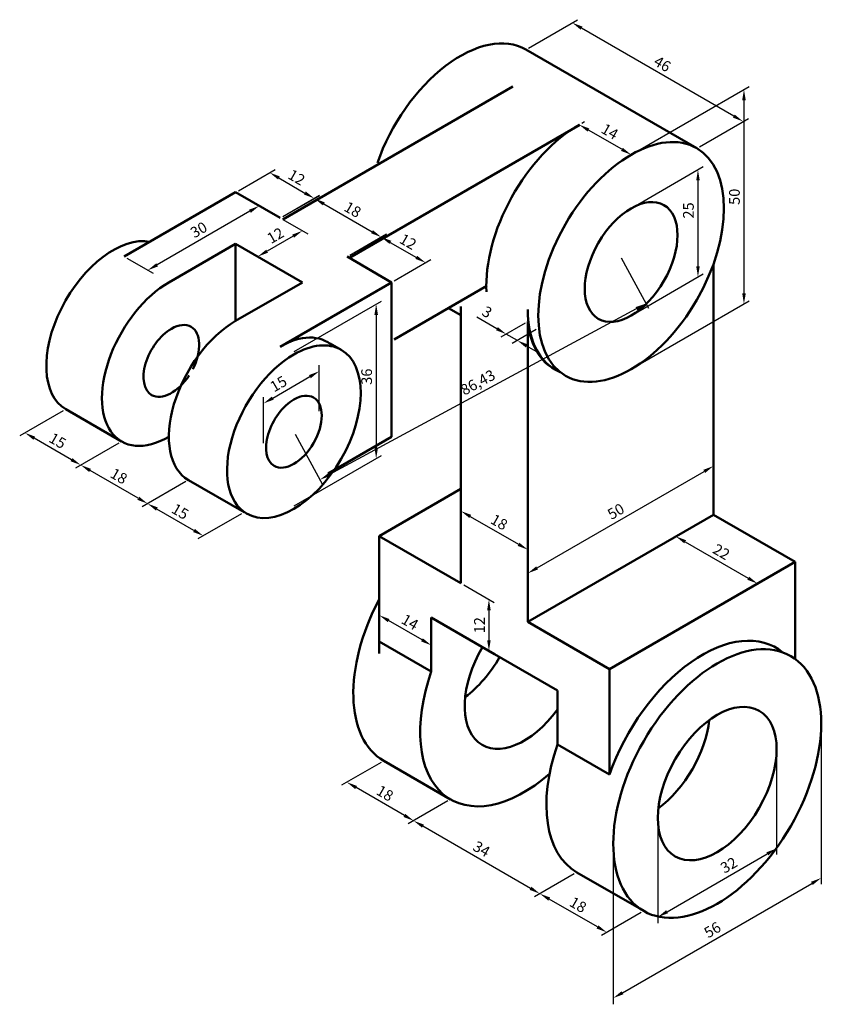
# Model space of a CAD drawing. Units: millimetres. Extents: x 2791 to 2981, y 1290 to 1520.
import ezdxf

# ---------------------------------------------------------------- set-up
doc = ezdxf.new("R2010")
doc.units = ezdxf.units.MM
doc.layers.add('M-DIMS', color=2, linetype='Continuous', lineweight=25)
doc.layers.add('M-OUTL', color=7, linetype='Continuous', lineweight=50)
doc.styles.get("Standard").update_dxf_attribs({"font": 'arial.ttf'})
doc.dimstyles.new('ISO-25', dxfattribs={"dimtxt": 2.5, "dimasz": 2.5, "dimexe": 1.25, "dimexo": 0.625, "dimtad": 1, "dimtxsty": 'Standard', "dimcen": 2.5, "dimadec": 0, "dimazin": 0, "dimtfac": 1, "dimtmove": 0, "dimatfit": 3, "dimfxl": 1, "dimarcsym": 0})

# ---------------------------------------------------------------- blocks, each defined once
blk = doc.blocks.new('*D1')
at = {"layer": 'Defpoints', "color": 0, "transparency": 16777216}
for p in [(2920.37, 1519.25), (2909.57, 1513.01), (2949.4, 1490.01)]:
    blk.add_point(p, dxfattribs=at)
at = {"layer": 'M-DIMS', "color": 0, "lineweight": -2, "transparency": 16777216}
for p, q in [((2910.19, 1513.37), (2921.62, 1519.97)), ((2958.04, 1497.5), (2922.53, 1518)), ((2950.03, 1490.37), (2961.45, 1496.97))]:
    blk.add_line(p, q, dxfattribs=at)
at = {"layer": 'M-DIMS', "color": 0, "transparency": 16777216}
for points in [[(2922.74, 1518.36), (2922.32, 1517.64), (2920.37, 1519.25)], [(2958.25, 1497.86), (2957.83, 1497.14), (2960.2, 1496.25)]]:
    blk.add_solid(points, dxfattribs=at)
at = {"layer": 'M-DIMS', "color": 0, "transparency": 16777216, "insert": (2941.23, 1509.39), "char_height": 2.5, "attachment_point": 5, "rotation": 330}
blk.add_mtext('46', dxfattribs=at)
blk = doc.blocks.new('*D2')
at = {"layer": 'Defpoints', "color": 0, "transparency": 16777216}
for p in [(2830.84, 1412.65), (2821.32, 1407.16), (2843.83, 1405.15)]:
    blk.add_point(p, dxfattribs=at)
at = {"layer": 'M-DIMS', "color": 0, "lineweight": -2, "transparency": 16777216}
for p, q in [((2830.21, 1412.29), (2820.07, 1406.43)), ((2832.14, 1400.91), (2823.48, 1405.91)), ((2843.2, 1404.79), (2833.06, 1398.93))]:
    blk.add_line(p, q, dxfattribs=at)
at = {"layer": 'M-DIMS', "color": 0, "transparency": 16777216}
for points in [[(2823.69, 1406.27), (2823.27, 1405.54), (2821.32, 1407.16)], [(2832.35, 1401.27), (2831.93, 1400.54), (2834.31, 1399.66)]]:
    blk.add_solid(points, dxfattribs=at)
at = {"layer": 'M-DIMS', "color": 0, "transparency": 16777216, "insert": (2828.76, 1405.05), "char_height": 2.5, "attachment_point": 5, "rotation": 330}
blk.add_mtext('15', dxfattribs=at)
blk = doc.blocks.new('*D3')
at = {"layer": 'Defpoints', "color": 0, "transparency": 16777216}
for p in [(2815.25, 1421.65), (2805.73, 1416.16), (2830.84, 1412.65)]:
    blk.add_point(p, dxfattribs=at)
at = {"layer": 'M-DIMS', "color": 0, "lineweight": -2, "transparency": 16777216}
for p, q in [((2814.63, 1421.29), (2804.48, 1415.43)), ((2819.15, 1408.41), (2807.89, 1414.91)), ((2830.21, 1412.29), (2820.07, 1406.43))]:
    blk.add_line(p, q, dxfattribs=at)
at = {"layer": 'M-DIMS', "color": 0, "transparency": 16777216}
for points in [[(2808.1, 1415.27), (2807.68, 1414.54), (2805.73, 1416.16)], [(2819.36, 1408.77), (2818.94, 1408.04), (2821.32, 1407.16)]]:
    blk.add_solid(points, dxfattribs=at)
at = {"layer": 'M-DIMS', "color": 0, "transparency": 16777216, "insert": (2814.47, 1413.3), "char_height": 2.5, "attachment_point": 5, "rotation": 330}
blk.add_mtext('18', dxfattribs=at)
blk = doc.blocks.new('*D4')
at = {"layer": 'Defpoints', "color": 0, "transparency": 16777216}
for p in [(2802.26, 1429.15), (2792.74, 1423.66), (2815.25, 1421.65)]:
    blk.add_point(p, dxfattribs=at)
at = {"layer": 'M-DIMS', "color": 0, "lineweight": -2, "transparency": 16777216}
for p, q in [((2801.63, 1428.79), (2791.49, 1422.93)), ((2803.56, 1417.41), (2794.9, 1422.41)), ((2814.63, 1421.29), (2804.48, 1415.43))]:
    blk.add_line(p, q, dxfattribs=at)
at = {"layer": 'M-DIMS', "color": 0, "transparency": 16777216}
for points in [[(2795.11, 1422.77), (2794.69, 1422.04), (2792.74, 1423.66)], [(2803.77, 1417.77), (2803.35, 1417.04), (2805.73, 1416.16)]]:
    blk.add_solid(points, dxfattribs=at)
at = {"layer": 'M-DIMS', "color": 0, "transparency": 16777216, "insert": (2800.18, 1421.55), "char_height": 2.5, "attachment_point": 5, "rotation": 330}
blk.add_mtext('15', dxfattribs=at)
blk = doc.blocks.new('*D5')
at = {"layer": 'Defpoints', "color": 0, "transparency": 16777216}
for p in [(2921.43, 1321.21), (2912.82, 1316.23), (2937.02, 1312.21)]:
    blk.add_point(p, dxfattribs=at)
at = {"layer": 'M-DIMS', "color": 0, "lineweight": -2, "transparency": 16777216}
for p, q in [((2920.81, 1320.85), (2911.57, 1315.51)), ((2926.24, 1308.48), (2914.99, 1314.98)), ((2936.4, 1311.85), (2927.16, 1306.51))]:
    blk.add_line(p, q, dxfattribs=at)
at = {"layer": 'M-DIMS', "color": 0, "transparency": 16777216}
for points in [[(2915.19, 1315.35), (2914.78, 1314.62), (2912.82, 1316.23)], [(2926.45, 1308.85), (2926.04, 1308.12), (2928.41, 1307.23)]]:
    blk.add_solid(points, dxfattribs=at)
at = {"layer": 'M-DIMS', "color": 0, "transparency": 16777216, "insert": (2921.57, 1313.38), "char_height": 2.5, "attachment_point": 5, "rotation": 330}
blk.add_mtext('18', dxfattribs=at)
blk = doc.blocks.new('*D6')
at = {"layer": 'Defpoints', "color": 0, "transparency": 16777216}
for p in [(2891.99, 1338.21), (2883.38, 1333.23), (2921.43, 1321.21)]:
    blk.add_point(p, dxfattribs=at)
at = {"layer": 'M-DIMS', "color": 0, "lineweight": -2, "transparency": 16777216}
for p, q in [((2891.36, 1337.85), (2882.13, 1332.51)), ((2910.66, 1317.48), (2885.54, 1331.98)), ((2920.81, 1320.85), (2911.57, 1315.51))]:
    blk.add_line(p, q, dxfattribs=at)
at = {"layer": 'M-DIMS', "color": 0, "transparency": 16777216}
for points in [[(2885.75, 1332.35), (2885.33, 1331.62), (2883.38, 1333.23)], [(2910.86, 1317.85), (2910.45, 1317.12), (2912.82, 1316.23)]]:
    blk.add_solid(points, dxfattribs=at)
at = {"layer": 'M-DIMS', "color": 0, "transparency": 16777216, "insert": (2899.05, 1326.38), "char_height": 2.5, "attachment_point": 5, "rotation": 330}
blk.add_mtext('34', dxfattribs=at)
blk = doc.blocks.new('*D7')
at = {"layer": 'Defpoints', "color": 0, "transparency": 16777216}
for p in [(2876.4, 1347.21), (2867.79, 1342.23), (2891.99, 1338.21)]:
    blk.add_point(p, dxfattribs=at)
at = {"layer": 'M-DIMS', "color": 0, "lineweight": -2, "transparency": 16777216}
for p, q in [((2875.77, 1346.85), (2866.54, 1341.51)), ((2881.21, 1334.48), (2869.95, 1340.98)), ((2891.36, 1337.85), (2882.13, 1332.51))]:
    blk.add_line(p, q, dxfattribs=at)
at = {"layer": 'M-DIMS', "color": 0, "transparency": 16777216}
for points in [[(2870.16, 1341.35), (2869.74, 1340.62), (2867.79, 1342.23)], [(2881.42, 1334.85), (2881, 1334.12), (2883.38, 1333.23)]]:
    blk.add_solid(points, dxfattribs=at)
at = {"layer": 'M-DIMS', "color": 0, "transparency": 16777216, "insert": (2876.53, 1339.38), "char_height": 2.5, "attachment_point": 5, "rotation": 330}
blk.add_mtext('18', dxfattribs=at)
blk = doc.blocks.new('*D8')
at = {"layer": 'Defpoints', "color": 0, "transparency": 16777216}
for p in [(2968.02, 1349.9), (2940.31, 1333.9), (2968.02, 1326.78)]:
    blk.add_point(p, dxfattribs=at)
at = {"layer": 'M-DIMS', "color": 0, "lineweight": -2, "transparency": 16777216}
for p, q in [((2968.02, 1349.18), (2968.02, 1325.34)), ((2940.31, 1333.18), (2940.31, 1309.34)), ((2942.48, 1312.03), (2965.86, 1325.53))]:
    blk.add_line(p, q, dxfattribs=at)
at = {"layer": 'M-DIMS', "color": 0, "transparency": 16777216}
for points in [[(2965.65, 1325.89), (2966.07, 1325.17), (2968.02, 1326.78)], [(2942.27, 1312.39), (2942.68, 1311.67), (2940.31, 1310.78)]]:
    blk.add_solid(points, dxfattribs=at)
at = {"layer": 'M-DIMS', "color": 0, "transparency": 16777216, "insert": (2957.04, 1322.63), "char_height": 2.5, "attachment_point": 5, "rotation": 30}
blk.add_mtext('32', dxfattribs=at)
blk = doc.blocks.new('*D9')
at = {"layer": 'Defpoints', "color": 0, "transparency": 16777216}
for p in [(2978.42, 1355.9), (2929.92, 1327.9), (2978.42, 1319.9)]:
    blk.add_point(p, dxfattribs=at)
at = {"layer": 'M-DIMS', "color": 0, "lineweight": -2, "transparency": 16777216}
for p, q in [((2978.42, 1355.18), (2978.42, 1318.45)), ((2929.92, 1327.18), (2929.92, 1290.45)), ((2932.08, 1293.15), (2976.25, 1318.65))]:
    blk.add_line(p, q, dxfattribs=at)
at = {"layer": 'M-DIMS', "color": 0, "transparency": 16777216}
for points in [[(2976.04, 1319.01), (2976.46, 1318.29), (2978.42, 1319.9)], [(2931.88, 1293.51), (2932.29, 1292.79), (2929.92, 1291.9)]]:
    blk.add_solid(points, dxfattribs=at)
at = {"layer": 'M-DIMS', "color": 0, "transparency": 16777216, "insert": (2953.22, 1307.54), "char_height": 2.5, "attachment_point": 5, "rotation": 30}
blk.add_mtext('56', dxfattribs=at)
blk = doc.blocks.new('*D10')
at = {"layer": 'Defpoints', "color": 0, "transparency": 16777216}
for p in [(2953.3, 1415.93), (2953.3, 1404.59), (2910, 1379.59)]:
    blk.add_point(p, dxfattribs=at)
at = {"layer": 'M-DIMS', "color": 0, "lineweight": -2, "transparency": 16777216}
for p, q in [((2953.3, 1405.31), (2953.3, 1417.37)), ((2912.17, 1392.18), (2951.14, 1414.68)), ((2910, 1380.31), (2910, 1392.37))]:
    blk.add_line(p, q, dxfattribs=at)
at = {"layer": 'M-DIMS', "color": 0, "transparency": 16777216}
for points in [[(2950.93, 1415.04), (2951.35, 1414.32), (2953.3, 1415.93)], [(2911.96, 1392.54), (2912.37, 1391.82), (2910, 1390.93)]]:
    blk.add_solid(points, dxfattribs=at)
at = {"layer": 'M-DIMS', "color": 0, "transparency": 16777216, "insert": (2930.7, 1405.08), "char_height": 2.5, "attachment_point": 5, "rotation": 30}
blk.add_mtext('50', dxfattribs=at)
blk = doc.blocks.new('*D11')
at = {"layer": 'Defpoints', "color": 0, "transparency": 16777216}
for p in [(2910, 1396.43), (2894.41, 1388.59), (2910, 1379.59)]:
    blk.add_point(p, dxfattribs=at)
at = {"layer": 'M-DIMS', "color": 0, "lineweight": -2, "transparency": 16777216}
for p, q in [((2894.41, 1389.31), (2894.41, 1406.87)), ((2896.58, 1404.18), (2907.84, 1397.68)), ((2910, 1380.31), (2910, 1397.87))]:
    blk.add_line(p, q, dxfattribs=at)
at = {"layer": 'M-DIMS', "color": 0, "transparency": 16777216}
for points in [[(2896.79, 1404.54), (2896.37, 1403.82), (2894.41, 1405.43)], [(2908.04, 1398.04), (2907.63, 1397.32), (2910, 1396.43)]]:
    blk.add_solid(points, dxfattribs=at)
at = {"layer": 'M-DIMS', "color": 0, "transparency": 16777216, "insert": (2903.16, 1402.58), "char_height": 2.5, "attachment_point": 5, "rotation": 330}
blk.add_mtext('18', dxfattribs=at)
blk = doc.blocks.new('*D12')
at = {"layer": 'Defpoints', "color": 0, "transparency": 16777216}
for p in [(2953.3, 1404.59), (2972.35, 1393.59), (2963.58, 1388.52)]:
    blk.add_point(p, dxfattribs=at)
at = {"layer": 'M-DIMS', "color": 0, "lineweight": -2, "transparency": 16777216}
for p, q in [((2952.68, 1404.22), (2943.27, 1398.8)), ((2946.69, 1398.27), (2961.41, 1389.77)), ((2971.73, 1393.22), (2962.33, 1387.8))]:
    blk.add_line(p, q, dxfattribs=at)
at = {"layer": 'M-DIMS', "color": 0, "transparency": 16777216}
for points in [[(2946.9, 1398.63), (2946.48, 1397.91), (2944.52, 1399.52)], [(2961.62, 1390.13), (2961.2, 1389.41), (2963.58, 1388.52)]]:
    blk.add_solid(points, dxfattribs=at)
at = {"layer": 'M-DIMS', "color": 0, "transparency": 16777216, "insert": (2954.99, 1395.65), "char_height": 2.5, "attachment_point": 5, "rotation": 330}
blk.add_mtext('22', dxfattribs=at)
blk = doc.blocks.new('*D13')
at = {"layer": 'Defpoints', "color": 0, "transparency": 16777216}
for p in [(2875.36, 1387.59), (2875.36, 1381.15), (2887.48, 1380.59)]:
    blk.add_point(p, dxfattribs=at)
at = {"layer": 'M-DIMS', "color": 0, "lineweight": -2, "transparency": 16777216}
for p, q in [((2875.36, 1386.86), (2875.36, 1379.71)), ((2885.32, 1375.4), (2877.52, 1379.9)), ((2887.48, 1379.86), (2887.48, 1372.71))]:
    blk.add_line(p, q, dxfattribs=at)
at = {"layer": 'M-DIMS', "color": 0, "transparency": 16777216}
for points in [[(2877.73, 1380.26), (2877.32, 1379.54), (2875.36, 1381.15)], [(2885.53, 1375.76), (2885.11, 1375.04), (2887.48, 1374.15)]]:
    blk.add_solid(points, dxfattribs=at)
at = {"layer": 'M-DIMS', "color": 0, "transparency": 16777216, "insert": (2882.36, 1379.28), "char_height": 2.5, "attachment_point": 5, "rotation": 330}
blk.add_mtext('14', dxfattribs=at)
blk = doc.blocks.new('*D14')
at = {"layer": 'Defpoints', "color": 0, "transparency": 16777216}
for p in [(2894.41, 1388.59), (2894.41, 1376.59), (2900.93, 1372.82)]:
    blk.add_point(p, dxfattribs=at)
at = {"layer": 'M-DIMS', "color": 0, "lineweight": -2, "transparency": 16777216}
for p, q in [((2895.04, 1388.22), (2902.18, 1384.1)), ((2900.93, 1382.32), (2900.93, 1375.32)), ((2895.04, 1376.22), (2902.18, 1372.1))]:
    blk.add_line(p, q, dxfattribs=at)
at = {"layer": 'M-DIMS', "color": 0, "transparency": 16777216}
for points in [[(2900.51, 1382.32), (2901.34, 1382.32), (2900.93, 1384.82)], [(2900.51, 1375.32), (2901.34, 1375.32), (2900.93, 1372.82)]]:
    blk.add_solid(points, dxfattribs=at)
at = {"layer": 'M-DIMS', "color": 0, "transparency": 16777216, "insert": (2899.05, 1378.82), "char_height": 2.5, "attachment_point": 5, "rotation": 90}
blk.add_mtext('12', dxfattribs=at)
blk = doc.blocks.new('*D15')
at = {"layer": 'Defpoints', "color": 0, "transparency": 16777216}
for p in [(2934.09, 1488.5), (2960.41, 1453.69), (2934.09, 1438.5)]:
    blk.add_point(p, dxfattribs=at)
at = {"layer": 'M-DIMS', "color": 0, "lineweight": -2, "transparency": 16777216}
for p, q in [((2934.72, 1488.86), (2961.66, 1504.41)), ((2960.41, 1501.19), (2960.41, 1456.19)), ((2934.72, 1438.86), (2961.66, 1454.41))]:
    blk.add_line(p, q, dxfattribs=at)
at = {"layer": 'M-DIMS', "color": 0, "transparency": 16777216}
for points in [[(2960, 1501.19), (2960.83, 1501.19), (2960.41, 1503.69)], [(2960, 1456.19), (2960.83, 1456.19), (2960.41, 1453.69)]]:
    blk.add_solid(points, dxfattribs=at)
at = {"layer": 'M-DIMS', "color": 0, "transparency": 16777216, "insert": (2958.51, 1478.69), "char_height": 2.5, "attachment_point": 5, "rotation": 90}
blk.add_mtext('50', dxfattribs=at)
blk = doc.blocks.new('*D16')
at = {"layer": 'Defpoints', "color": 0, "transparency": 16777216}
for p in [(2934.09, 1476), (2949.68, 1460), (2934.09, 1451)]:
    blk.add_point(p, dxfattribs=at)
at = {"layer": 'M-DIMS', "color": 0, "lineweight": -2, "transparency": 16777216}
for p, q in [((2934.72, 1476.36), (2950.93, 1485.72)), ((2949.68, 1482.5), (2949.68, 1462.5)), ((2934.72, 1451.36), (2950.93, 1460.72))]:
    blk.add_line(p, q, dxfattribs=at)
at = {"layer": 'M-DIMS', "color": 0, "transparency": 16777216}
for points in [[(2949.27, 1482.5), (2950.1, 1482.5), (2949.68, 1485)], [(2949.27, 1462.5), (2950.1, 1462.5), (2949.68, 1460)]]:
    blk.add_solid(points, dxfattribs=at)
at = {"layer": 'M-DIMS', "color": 0, "transparency": 16777216, "insert": (2947.78, 1475.5), "char_height": 2.5, "attachment_point": 5, "rotation": 90}
blk.add_mtext('25', dxfattribs=at)
blk = doc.blocks.new('*D17')
at = {"layer": 'Defpoints', "color": 0, "transparency": 16777216}
for p in [(2867.84, 1464.75), (2886.16, 1463.32), (2878.23, 1458.75)]:
    blk.add_point(p, dxfattribs=at)
at = {"layer": 'M-DIMS', "color": 0, "lineweight": -2, "transparency": 16777216}
for p, q in [((2868.47, 1465.11), (2877.02, 1470.04)), ((2877.93, 1468.07), (2884, 1464.57)), ((2878.86, 1459.11), (2887.41, 1464.04))]:
    blk.add_line(p, q, dxfattribs=at)
at = {"layer": 'M-DIMS', "color": 0, "transparency": 16777216}
for points in [[(2878.14, 1468.43), (2877.73, 1467.71), (2875.77, 1469.32)], [(2884.2, 1464.93), (2883.79, 1464.21), (2886.16, 1463.32)]]:
    blk.add_solid(points, dxfattribs=at)
at = {"layer": 'M-DIMS', "color": 0, "transparency": 16777216, "insert": (2881.91, 1467.95), "char_height": 2.5, "attachment_point": 5, "rotation": 330}
blk.add_mtext('12', dxfattribs=at)
blk = doc.blocks.new('*D18')
at = {"layer": 'Defpoints', "color": 0, "transparency": 16777216}
for p in [(2852.32, 1473.7), (2875.84, 1469.28), (2867.91, 1464.7)]:
    blk.add_point(p, dxfattribs=at)
at = {"layer": 'M-DIMS', "color": 0, "lineweight": -2, "transparency": 16777216}
for p, q in [((2852.95, 1474.07), (2861.5, 1479)), ((2862.42, 1477.03), (2873.67, 1470.53)), ((2868.54, 1465.07), (2877.09, 1470))]:
    blk.add_line(p, q, dxfattribs=at)
at = {"layer": 'M-DIMS', "color": 0, "transparency": 16777216}
for points in [[(2862.62, 1477.39), (2862.21, 1476.67), (2860.25, 1478.28)], [(2873.88, 1470.89), (2873.47, 1470.17), (2875.84, 1469.28)]]:
    blk.add_solid(points, dxfattribs=at)
at = {"layer": 'M-DIMS', "color": 0, "transparency": 16777216, "insert": (2869, 1475.43), "char_height": 2.5, "attachment_point": 5, "rotation": 330}
blk.add_mtext('18', dxfattribs=at)
blk = doc.blocks.new('*D19')
at = {"layer": 'Defpoints', "color": 0, "transparency": 16777216}
for p in [(2841.86, 1479.75), (2860.18, 1478.32), (2852.25, 1473.75)]:
    blk.add_point(p, dxfattribs=at)
at = {"layer": 'M-DIMS', "color": 0, "lineweight": -2, "transparency": 16777216}
for p, q in [((2842.49, 1480.11), (2851.04, 1485.04)), ((2851.95, 1483.07), (2858.02, 1479.57)), ((2852.88, 1474.11), (2861.43, 1479.04))]:
    blk.add_line(p, q, dxfattribs=at)
at = {"layer": 'M-DIMS', "color": 0, "transparency": 16777216}
for points in [[(2852.16, 1483.43), (2851.75, 1482.71), (2849.79, 1484.32)], [(2858.22, 1479.93), (2857.81, 1479.21), (2860.18, 1478.32)]]:
    blk.add_solid(points, dxfattribs=at)
at = {"layer": 'M-DIMS', "color": 0, "transparency": 16777216, "insert": (2855.92, 1482.95), "char_height": 2.5, "attachment_point": 5, "rotation": 330}
blk.add_mtext('12', dxfattribs=at)
blk = doc.blocks.new('*D20')
at = {"layer": 'Defpoints', "color": 0, "transparency": 16777216}
for p in [(2852.25, 1473.75), (2841.86, 1467.75), (2847.03, 1464.76)]:
    blk.add_point(p, dxfattribs=at)
at = {"layer": 'M-DIMS', "color": 0, "lineweight": -2, "transparency": 16777216}
for p, q in [((2852.88, 1473.38), (2858.67, 1470.04)), ((2855.26, 1469.51), (2849.2, 1466.01)), ((2842.49, 1467.38), (2848.28, 1464.04))]:
    blk.add_line(p, q, dxfattribs=at)
at = {"layer": 'M-DIMS', "color": 0, "transparency": 16777216}
for points in [[(2855.05, 1469.87), (2855.47, 1469.15), (2857.42, 1470.76)], [(2848.99, 1466.37), (2849.4, 1465.65), (2847.03, 1464.76)]]:
    blk.add_solid(points, dxfattribs=at)
at = {"layer": 'M-DIMS', "color": 0, "transparency": 16777216, "insert": (2851.29, 1469.39), "char_height": 2.5, "attachment_point": 5, "rotation": 30}
blk.add_mtext('12', dxfattribs=at)
blk = doc.blocks.new('*D21')
at = {"layer": 'Defpoints', "color": 0, "transparency": 16777216}
for p in [(2841.86, 1479.75), (2815.88, 1464.75), (2821.37, 1461.57)]:
    blk.add_point(p, dxfattribs=at)
at = {"layer": 'M-DIMS', "color": 0, "lineweight": -2, "transparency": 16777216}
for p, q in [((2842.49, 1479.38), (2848.6, 1475.85)), ((2845.19, 1475.32), (2823.54, 1462.82)), ((2816.51, 1464.38), (2822.62, 1460.85))]:
    blk.add_line(p, q, dxfattribs=at)
at = {"layer": 'M-DIMS', "color": 0, "transparency": 16777216}
for points in [[(2844.98, 1475.68), (2845.4, 1474.96), (2847.35, 1476.57)], [(2823.33, 1463.18), (2823.75, 1462.46), (2821.37, 1461.57)]]:
    blk.add_solid(points, dxfattribs=at)
at = {"layer": 'M-DIMS', "color": 0, "transparency": 16777216, "insert": (2833.41, 1470.72), "char_height": 2.5, "attachment_point": 5, "rotation": 30}
blk.add_mtext('30', dxfattribs=at)
blk = doc.blocks.new('*D22')
at = {"layer": 'Defpoints', "color": 0, "transparency": 16777216}
for p in [(2861.35, 1438.02), (2861.35, 1428), (2848.36, 1420.5)]:
    blk.add_point(p, dxfattribs=at)
at = {"layer": 'M-DIMS', "color": 0, "lineweight": -2, "transparency": 16777216}
for p, q in [((2861.35, 1428.72), (2861.35, 1439.46)), ((2850.52, 1431.77), (2859.18, 1436.77)), ((2848.36, 1421.22), (2848.36, 1431.96))]:
    blk.add_line(p, q, dxfattribs=at)
at = {"layer": 'M-DIMS', "color": 0, "transparency": 16777216}
for points in [[(2858.97, 1437.13), (2859.39, 1436.4), (2861.35, 1438.02)], [(2850.31, 1432.13), (2850.73, 1431.4), (2848.36, 1430.52)]]:
    blk.add_solid(points, dxfattribs=at)
at = {"layer": 'M-DIMS', "color": 0, "transparency": 16777216, "insert": (2852, 1434.81), "char_height": 2.5, "attachment_point": 5, "rotation": 30}
blk.add_mtext('15', dxfattribs=at)
blk = doc.blocks.new('*D23')
at = {"layer": 'Defpoints', "color": 0, "transparency": 16777216}
for p in [(2854.85, 1442.25), (2874.63, 1417.67), (2854.85, 1406.25)]:
    blk.add_point(p, dxfattribs=at)
at = {"layer": 'M-DIMS', "color": 0, "lineweight": -2, "transparency": 16777216}
for p, q in [((2855.48, 1442.61), (2875.88, 1454.39)), ((2874.63, 1451.17), (2874.63, 1420.17)), ((2855.48, 1406.61), (2875.88, 1418.39))]:
    blk.add_line(p, q, dxfattribs=at)
at = {"layer": 'M-DIMS', "color": 0, "transparency": 16777216}
for points in [[(2874.22, 1451.17), (2875.05, 1451.17), (2874.63, 1453.67)], [(2874.22, 1420.17), (2875.05, 1420.17), (2874.63, 1417.67)]]:
    blk.add_solid(points, dxfattribs=at)
at = {"layer": 'M-DIMS', "color": 0, "transparency": 16777216, "insert": (2872.73, 1436.76), "char_height": 2.5, "attachment_point": 5, "rotation": 90}
blk.add_mtext('36', dxfattribs=at)
blk = doc.blocks.new('*D24')
at = {"layer": 'Defpoints', "color": 0, "transparency": 16777216}
for p in [(2910, 1449.59), (2904.97, 1446.68), (2912.6, 1448.09)]:
    blk.add_point(p, dxfattribs=at)
at = {"layer": 'M-DIMS', "color": 0, "lineweight": -2, "transparency": 16777216}
for p, q in [((2902.8, 1447.93), (2898.14, 1450.62)), ((2909.38, 1449.22), (2903.72, 1445.96)), ((2907.57, 1445.18), (2904.97, 1446.68)), ((2911.97, 1447.72), (2906.32, 1444.46)), ((2909.73, 1443.93), (2911.9, 1442.68))]:
    blk.add_line(p, q, dxfattribs=at)
at = {"layer": 'M-DIMS', "color": 0, "transparency": 16777216}
for points in [[(2903.01, 1448.29), (2902.59, 1447.57), (2904.97, 1446.68)], [(2909.94, 1444.29), (2909.52, 1443.57), (2907.57, 1445.18)]]:
    blk.add_solid(points, dxfattribs=at)
at = {"layer": 'M-DIMS', "color": 0, "transparency": 16777216, "insert": (2900.34, 1451.55), "char_height": 2.5, "attachment_point": 5, "rotation": 330}
blk.add_mtext('3', dxfattribs=at)
blk = doc.blocks.new('*D25')
at = {"layer": 'Defpoints', "color": 0, "transparency": 16777216}
for p in [(2921.97, 1495.5), (2921.97, 1495.5), (2934.09, 1488.5)]:
    blk.add_point(p, dxfattribs=at)
at = {"layer": 'M-DIMS', "color": 0, "lineweight": -2, "transparency": 16777216}
for p, q in [((2922.59, 1495.86), (2923.22, 1496.22)), ((2931.93, 1489.75), (2924.13, 1494.25)), ((2934.72, 1488.86), (2935.34, 1489.22))]:
    blk.add_line(p, q, dxfattribs=at)
at = {"layer": 'M-DIMS', "color": 0, "transparency": 16777216}
for points in [[(2924.34, 1494.61), (2923.93, 1493.88), (2921.97, 1495.5)], [(2932.14, 1490.11), (2931.72, 1489.38), (2934.09, 1488.5)]]:
    blk.add_solid(points, dxfattribs=at)
at = {"layer": 'M-DIMS', "color": 0, "transparency": 16777216, "insert": (2928.97, 1493.62), "char_height": 2.5, "attachment_point": 5, "rotation": 330}
blk.add_mtext('14', dxfattribs=at)
blk = doc.blocks.new('*D26')
at = {"layer": 'Defpoints', "color": 0, "transparency": 16777216}
for p in [(2931.49, 1465), (2937.54, 1453.8), (2855.44, 1423.93)]:
    blk.add_point(p, dxfattribs=at)
at = {"layer": 'M-DIMS', "color": 0, "lineweight": -2, "transparency": 16777216}
for p, q in [((2931.79, 1464.45), (2938.14, 1452.7)), ((2863.69, 1413.92), (2935.34, 1452.61)), ((2855.74, 1423.38), (2862.08, 1411.63))]:
    blk.add_line(p, q, dxfattribs=at)
at = {"layer": 'M-DIMS', "color": 0, "transparency": 16777216}
for points in [[(2935.14, 1452.97), (2935.54, 1452.24), (2937.54, 1453.8)], [(2863.49, 1414.29), (2863.88, 1413.55), (2861.49, 1412.73)]]:
    blk.add_solid(points, dxfattribs=at)
at = {"layer": 'M-DIMS', "color": 0, "transparency": 16777216, "insert": (2898.5, 1435.14), "char_height": 2.5, "attachment_point": 5, "rotation": 28.3662}
blk.add_mtext('86,43', dxfattribs=at)

msp = doc.modelspace()

# ---------------------------------------------------------------- linework, layer by layer
at = {"layer": 'M-OUTL'}
for p, q in [((2949.402, 1490.012), (2909.565, 1513.012)), ((2852.841, 1473.43), (2906.535, 1504.43)), ((2868.43, 1464.43), (2922.123, 1495.43)), ((2815.88, 1464.745), (2841.861, 1479.745)), ((2841.861, 1479.745), (2852.254, 1473.745)), ((2826.273, 1458.745), (2841.861, 1467.745)), ((2857.45, 1458.745), (2841.861, 1467.745)), ((2841.861, 1467.745), (2841.861, 1449.745)), ((2867.842, 1464.745), (2878.234, 1458.745)), ((2953.302, 1404.585), (2953.302, 1463.052)), ((2857.45, 1458.745), (2841.861, 1449.745)), ((2878.234, 1458.745), (2852.254, 1443.745)), ((2878.234, 1458.745), (2878.234, 1422.745)), ((2878.822, 1445.43), (2900.473, 1457.93)), ((2894.412, 1388.585), (2894.412, 1453.085)), ((2894.411, 1451.075), (2891.505, 1452.752)), ((2910.001, 1449.585), (2910.001, 1379.585)), ((2866.462, 1443.022), (2863.864, 1444.522)), ((2815.25, 1421.653), (2802.26, 1429.153)), ((2878.234, 1422.745), (2863.468, 1414.22)), ((2843.829, 1405.153), (2830.839, 1412.653)), ((2875.36, 1399.585), (2894.412, 1410.585)), ((2910.001, 1379.585), (2953.302, 1404.585)), ((2972.355, 1393.585), (2953.302, 1404.585)), ((2894.412, 1388.585), (2875.36, 1399.585)), ((2875.36, 1399.585), (2875.36, 1372.195)), ((2929.053, 1368.585), (2972.355, 1393.585)), ((2972.355, 1393.585), (2972.355, 1370.925)), ((2902.206, 1372.085), (2887.484, 1380.585)), ((2887.484, 1380.585), (2887.484, 1368.014)), ((2910.001, 1379.585), (2929.053, 1368.585)), ((2887.482, 1368.04), (2875.358, 1375.04)), ((2902.206, 1372.085), (2916.929, 1363.585)), ((2929.053, 1368.585), (2929.053, 1344.014)), ((2916.929, 1363.585), (2916.929, 1351.014)), ((2916.929, 1351.014), (2929.053, 1344.014)), ((2891.988, 1338.206), (2876.4, 1347.206)), ((2937.022, 1312.206), (2921.433, 1321.206))]:
    msp.add_line(p, q, dxfattribs=at)
for centre, major_axis, start_param, end_param in [((2894.256, 1486.495), (-15.309, -26.517), 3.1415927, 5.0312987), ((2921.969, 1470.495), (-15.309, -26.517), 3.9269908, 5.5578232), ((2931.495, 1464.995), (-15.309, -26.517), 3.0566377, 3.1415927), ((2813.282, 1448.245), (-11.023, -19.092), 3.3413053, 6.2831853), ((2826.273, 1440.745), (-11.023, -19.092), 3.9269908, 7.0685835), ((2931.65, 1464.93), (15.309, 26.517), 2.3561945, 3.1415927), ((2841.861, 1431.745), (-11.023, -19.092), 3.9269908, 6.2831853), ((2826.861, 1440.43), (4.593, 7.955), 0, 0.7853982), ((2826.861, 1440.43), (4.593, 7.955), 4.8036122, 6.2831853), ((2931.495, 1464.995), (-15.309, -26.517), 5.618077, 6.3681403), ((2826.861, 1440.43), (4.593, 7.955), 0.7853982, 3.1415927), ((2852.254, 1425.745), (-11.023, -19.092), 3.023467, 3.9269908), ((2855.439, 1423.93), (11.023, 19.092), 0, 0.7853982), ((2855.439, 1423.93), (11.023, 19.092), 0.7853982, 3.1415927), ((2855.439, 1423.93), (11.023, 19.092), 3.1415927, 6.2831853), ((2826.861, 1440.43), (4.593, 7.955), 3.1415927, 4.6211658), ((2855.439, 1423.93), (4.593, 7.955), 0, 0.7853982), ((2855.439, 1423.93), (4.593, 7.955), 0.7853982, 3.1415927), ((2855.439, 1423.93), (4.593, 7.955), 3.1415927, 6.2831853), ((2893.546, 1376.905), (-17.146, -29.698), 4.7750529, 6.2831853), ((2950.704, 1343.905), (-17.146, -29.698), 3.0404048, 5.030641), ((2909.135, 1367.905), (-9.798, -16.971), 4.7044051, 7.6659899), ((2893.546, 1376.905), (-9.798, -16.971), 0.9198242, 1.5787802), ((2909.135, 1367.905), (-17.146, -29.698), 5.030641, 7.3157756), ((2938.58, 1350.905), (-9.798, -16.971), 0.9198242, 2.2217684), ((2938.58, 1350.905), (-17.146, -29.698), 5.030641, 6.2831853)]:
    msp.add_ellipse(centre, major_axis=major_axis, ratio=0.5773503, start_param=start_param, end_param=end_param, dxfattribs=at)
for centre, major_axis in [((2934.093, 1463.495), (-15.309, -26.517)), ((2934.093, 1463.495), (-7.655, -13.258)), ((2954.168, 1341.905), (-17.146, -29.698)), ((2954.168, 1341.905), (-9.798, -16.971))]:
    msp.add_ellipse(centre, major_axis=major_axis, ratio=0.5773503, dxfattribs=at)

# ---------------------------------------------------------------- dimensions: what is measured, and where the dimension line sits
at = {"layer": 'M-DIMS'}
for p1, p2, distance, picture, middle in [((2949.402, 1490.012), (2909.565, 1513.012), -10.8, '*D1', (2941.235, 1509.394)), ((2934.093, 1488.495), (2934.093, 1438.495), 26.32, '*D15', (2958.512, 1478.691)), ((2934.093, 1488.495), (2921.969, 1495.495), 0, '*D25', (2928.971, 1493.623)), ((2841.861, 1479.745), (2852.254, 1473.745), 7.927, '*D19', (2855.925, 1482.95)), ((2841.861, 1479.745), (2815.88, 1464.745), 5.493, '*D21', (2833.413, 1470.721)), ((2852.324, 1473.705), (2867.912, 1464.705), 7.927, '*D18', (2868.996, 1475.428)), ((2852.254, 1473.745), (2841.861, 1467.745), 5.169, '*D20', (2851.287, 1469.389)), ((2867.842, 1464.745), (2878.234, 1458.745), 7.927, '*D17', (2881.906, 1467.95)), ((2815.25, 1421.653), (2802.26, 1429.153), 9.522, '*D4', (2800.184, 1421.552)), ((2830.839, 1412.653), (2815.25, 1421.653), 9.522, '*D3', (2814.473, 1413.302)), ((2910.001, 1379.585), (2953.302, 1404.585), 9.823, '*D10', (2930.701, 1405.075)), ((2843.829, 1405.153), (2830.839, 1412.653), 9.522, '*D2', (2828.762, 1405.052)), ((2894.412, 1388.585), (2910.001, 1379.585), 14.587, '*D11', (2903.157, 1402.576)), ((2953.302, 1404.585), (2972.355, 1393.585), -8.778, '*D12', (2954.99, 1395.646)), ((2894.412, 1388.585), (2894.412, 1376.585), 6.514, '*D14', (2899.046, 1378.825)), ((2887.484, 1380.585), (2875.36, 1387.585), 5.573, '*D13', (2882.362, 1379.279)), ((2891.988, 1338.206), (2876.4, 1347.206), 8.612, '*D7', (2876.533, 1339.381)), ((2921.433, 1321.206), (2891.988, 1338.206), 8.612, '*D6', (2899.05, 1326.382)), ((2937.022, 1312.206), (2921.433, 1321.206), 8.612, '*D5', (2921.566, 1313.381))]:
    dim = msp.add_aligned_dim(p1=p1, p2=p2, distance=distance, dimstyle='ISO-25', override={"dimclrd": 0, "dimclre": 0, "dimclrt": 0}, dxfattribs=at)
    dim.commit()
    dim.dimension.update_dxf_attribs({"geometry": picture, "text_midpoint": middle})
for base, p1, p2, angle, picture, middle in [((2949.683, 1459.996), (2934.093, 1475.995), (2934.093, 1450.995), 270, '*D16', (2949.683, 1475.503)), ((2874.633, 1417.666), (2854.852, 1442.245), (2854.852, 1406.245), 270, '*D23', (2874.633, 1436.764)), ((2904.968, 1446.68), (2912.599, 1448.085), (2910.001, 1449.585), 150, '*D24', (2899.388, 1449.902)), ((2861.347, 1438.016), (2848.356, 1420.495), (2861.347, 1427.995), 30, '*D22', (2852.95, 1433.168)), ((2978.417, 1319.897), (2929.919, 1327.905), (2978.417, 1355.905), 30, '*D9', (2954.168, 1305.897)), ((2968.024, 1326.78), (2940.312, 1333.905), (2968.024, 1349.905), 30, '*D8', (2957.99, 1320.986))]:
    dim = msp.add_linear_dim(base=base, p1=p1, p2=p2, angle=angle, dimstyle='ISO-25', override={"dimclrd": 0, "dimclre": 0, "dimclrt": 0}, dxfattribs=at)
    dim.commit()
    dim.dimension.update_dxf_attribs({"geometry": picture, "text_midpoint": middle, "dimtype": 161})
dim = msp.add_linear_dim(base=(2937.542, 1453.796), p1=(2855.439, 1423.93), p2=(2931.495, 1464.995), angle=28.3662, dimstyle='ISO-25', override={"dimrnd": 0}, dxfattribs=at)
dim.commit()
dim.dimension.update_dxf_attribs({"geometry": '*D26', "text_midpoint": (2898.503, 1435.135)})

doc.saveas('drawing.dxf')
